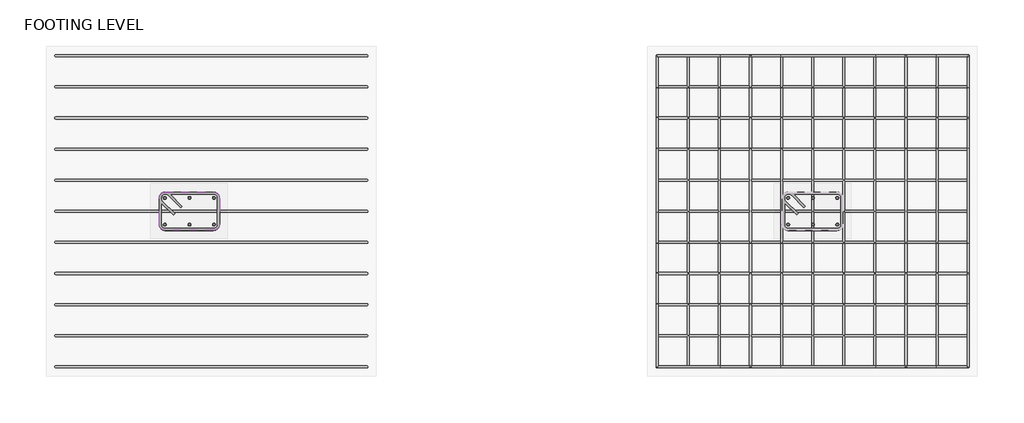
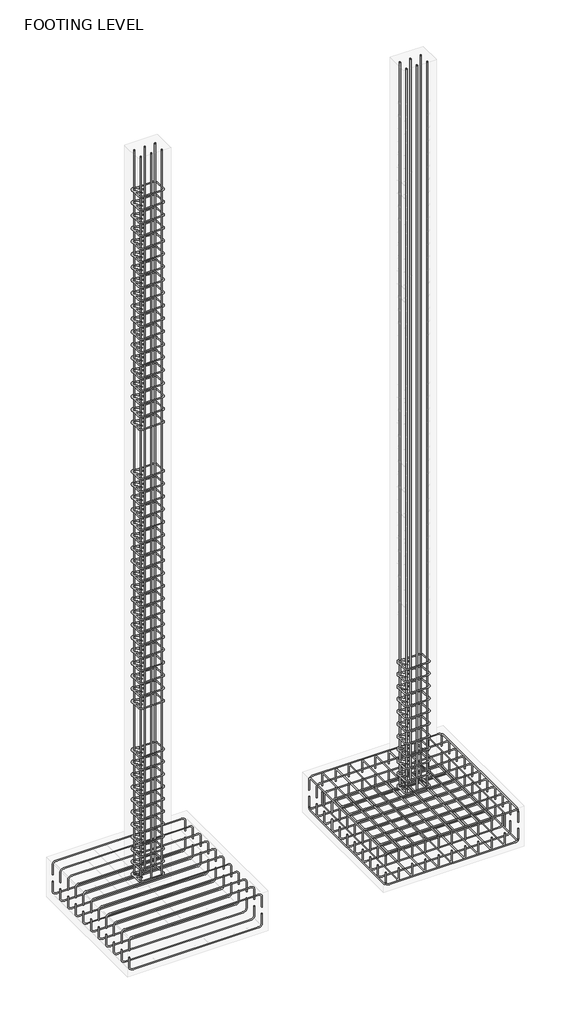
# One storey, part 8 of 9: 22 reinforcing bars.
"""IFC4 building model written with IfcOpenShell, lengths in millimetres."""

from ifc_helpers import new_model, si_unit, point, frame, origin, place, context, project, spatial, polyline, circle_curve, trimmed, segment, composite_curve, source, transform, mapped, element, save
from ifc_brep_helpers import swept_disk

model = new_model("IFC4")

# Units and contexts
model_context = context("Model", 3, world=origin())
ifc_project = project(units=[si_unit("LENGTHUNIT", "METRE", prefix="MILLI")], contexts=[model_context])

# Site, building, storey
site = spatial("IfcSite", under=ifc_project)
building = spatial("IfcBuilding", under=site)
storey = spatial("IfcBuildingStorey", under=building, Name="FOOTING LEVEL", Elevation=-1981.2)

# Reinforcing bars
placement = place(None, origin())
reinforcing_bar_shape = source(origin(), model_context, "Body", "SolidModel", [
    swept_disk(composite_curve([segment(polyline([(-6807.4208659, 8895.7158402, -2171.7), (-6807.4208659, 8895.7158402, -2057.4)]), True, "CONTINUOUS"), segment(trimmed(circle_curve(frame((-6774.0833659, 8895.7158402, -2057.4), z_axis=(0.0, 1.0, 0.0), x_axis=(-33.337499999999636, 0.0, 0.0)), 33.3375), [point((-6807.4208659, 8895.7158402, -2057.4))], [point((-6774.0833659, 8895.7158402, -2024.0625))], True, "CARTESIAN"), True, "CONTINUOUS"), segment(polyline([(-6774.0833659, 8895.7158402, -2024.0625), (-5402.4833659, 8895.7158402, -2024.0625)]), True, "CONTINUOUS"), segment(trimmed(circle_curve(frame((-5402.4833659, 8895.7158402, -2057.4), z_axis=(0.0, 1.0, 0.0), x_axis=(0.0, 0.0, 33.33750000000009)), 33.3375), [point((-5402.4833659, 8895.7158402, -2024.0625))], [point((-5369.1458659, 8895.7158402, -2057.4))], True, "CARTESIAN"), True, "CONTINUOUS"), segment(polyline([(-5369.1458659, 8895.7158402, -2057.4), (-5369.1458659, 8895.7158402, -2171.7)]), True, "CONTINUOUS")], self_intersect=False), 4.7625),
])
element("IfcReinforcingBar", 1, at=placement, inside=storey, context=model_context, shape_type="MappedRepresentation", body=[
    mapped(reinforcing_bar_shape, transform((0.0, 0.0, 0.0), x_axis=(1.0, 0.0, 0.0), y_axis=(0.0, 1.0, 0.0), z_axis=(0.0, 0.0, 1.0))),
    mapped(reinforcing_bar_shape, transform((0.0, -143.8275, 0.0), x_axis=(1.0, 0.0, 0.0), y_axis=(0.0, 1.0, 0.0), z_axis=(0.0, 0.0, 1.0))),
    mapped(reinforcing_bar_shape, transform((0.0, -287.655, 0.0), x_axis=(1.0, 0.0, 0.0), y_axis=(0.0, 1.0, 0.0), z_axis=(0.0, 0.0, 1.0))),
    mapped(reinforcing_bar_shape, transform((0.0, -431.4825, 0.0), x_axis=(1.0, 0.0, 0.0), y_axis=(0.0, 1.0, 0.0), z_axis=(0.0, 0.0, 1.0))),
    mapped(reinforcing_bar_shape, transform((0.0, -575.31, 0.0), x_axis=(1.0, 0.0, 0.0), y_axis=(0.0, 1.0, 0.0), z_axis=(0.0, 0.0, 1.0))),
    mapped(reinforcing_bar_shape, transform((0.0, -719.1375, 0.0), x_axis=(1.0, 0.0, 0.0), y_axis=(0.0, 1.0, 0.0), z_axis=(0.0, 0.0, 1.0))),
    mapped(reinforcing_bar_shape, transform((0.0, -862.965, 0.0), x_axis=(1.0, 0.0, 0.0), y_axis=(0.0, 1.0, 0.0), z_axis=(0.0, 0.0, 1.0))),
    mapped(reinforcing_bar_shape, transform((0.0, -1006.7925, 0.0), x_axis=(1.0, 0.0, 0.0), y_axis=(0.0, 1.0, 0.0), z_axis=(0.0, 0.0, 1.0))),
    mapped(reinforcing_bar_shape, transform((0.0, -1150.62, 0.0), x_axis=(1.0, 0.0, 0.0), y_axis=(0.0, 1.0, 0.0), z_axis=(0.0, 0.0, 1.0))),
    mapped(reinforcing_bar_shape, transform((0.0, -1294.4475, 0.0), x_axis=(1.0, 0.0, 0.0), y_axis=(0.0, 1.0, 0.0), z_axis=(0.0, 0.0, 1.0))),
    mapped(reinforcing_bar_shape, transform((0.0, -1438.275, 0.0), x_axis=(1.0, 0.0, 0.0), y_axis=(0.0, 1.0, 0.0), z_axis=(0.0, 0.0, 1.0))),
])
reinforcing_bar_2_shape = source(origin(), model_context, "Body", "SolidModel", [
    swept_disk(composite_curve([segment(polyline([(-6807.4208659, 7457.4408402, -2247.9), (-6807.4208659, 7457.4408402, -2362.2)]), True, "CONTINUOUS"), segment(trimmed(circle_curve(frame((-6774.0833659, 7457.4408402, -2362.2), z_axis=(0.0, -1.0, 0.0), x_axis=(-33.337499999999636, 0.0, 0.0)), 33.3375), [point((-6807.4208659, 7457.4408402, -2362.2))], [point((-6774.0833659, 7457.4408402, -2395.5375))], True, "CARTESIAN"), True, "CONTINUOUS"), segment(polyline([(-6774.0833659, 7457.4408402, -2395.5375), (-5402.4833659, 7457.4408402, -2395.5375)]), True, "CONTINUOUS"), segment(trimmed(circle_curve(frame((-5402.4833659, 7457.4408402, -2362.2), z_axis=(0.0, -1.0, 0.0), x_axis=(0.0, 0.0, -33.33750000000009)), 33.3375), [point((-5402.4833659, 7457.4408402, -2395.5375))], [point((-5369.1458659, 7457.4408402, -2362.2))], True, "CARTESIAN"), True, "CONTINUOUS"), segment(polyline([(-5369.1458659, 7457.4408402, -2362.2), (-5369.1458659, 7457.4408402, -2247.9)]), True, "CONTINUOUS")], self_intersect=False), 4.7625),
])
element("IfcReinforcingBar", 2, at=placement, inside=storey, context=model_context, shape_type="MappedRepresentation", body=[
    mapped(reinforcing_bar_2_shape, transform((0.0, 0.0, 0.0), x_axis=(1.0, 0.0, 0.0), y_axis=(0.0, 1.0, 0.0), z_axis=(0.0, 0.0, 1.0))),
    mapped(reinforcing_bar_2_shape, transform((0.0, 143.8275, 0.0), x_axis=(1.0, 0.0, 0.0), y_axis=(0.0, 1.0, 0.0), z_axis=(0.0, 0.0, 1.0))),
    mapped(reinforcing_bar_2_shape, transform((0.0, 287.655, 0.0), x_axis=(1.0, 0.0, 0.0), y_axis=(0.0, 1.0, 0.0), z_axis=(0.0, 0.0, 1.0))),
    mapped(reinforcing_bar_2_shape, transform((0.0, 431.4825, 0.0), x_axis=(1.0, 0.0, 0.0), y_axis=(0.0, 1.0, 0.0), z_axis=(0.0, 0.0, 1.0))),
    mapped(reinforcing_bar_2_shape, transform((0.0, 575.31, 0.0), x_axis=(1.0, 0.0, 0.0), y_axis=(0.0, 1.0, 0.0), z_axis=(0.0, 0.0, 1.0))),
    mapped(reinforcing_bar_2_shape, transform((0.0, 719.1375, 0.0), x_axis=(1.0, 0.0, 0.0), y_axis=(0.0, 1.0, 0.0), z_axis=(0.0, 0.0, 1.0))),
    mapped(reinforcing_bar_2_shape, transform((0.0, 862.965, 0.0), x_axis=(1.0, 0.0, 0.0), y_axis=(0.0, 1.0, 0.0), z_axis=(0.0, 0.0, 1.0))),
    mapped(reinforcing_bar_2_shape, transform((0.0, 1006.7925, 0.0), x_axis=(1.0, 0.0, 0.0), y_axis=(0.0, 1.0, 0.0), z_axis=(0.0, 0.0, 1.0))),
    mapped(reinforcing_bar_2_shape, transform((0.0, 1150.62, 0.0), x_axis=(1.0, 0.0, 0.0), y_axis=(0.0, 1.0, 0.0), z_axis=(0.0, 0.0, 1.0))),
    mapped(reinforcing_bar_2_shape, transform((0.0, 1294.4475, 0.0), x_axis=(1.0, 0.0, 0.0), y_axis=(0.0, 1.0, 0.0), z_axis=(0.0, 0.0, 1.0))),
    mapped(reinforcing_bar_2_shape, transform((0.0, 1438.275, 0.0), x_axis=(1.0, 0.0, 0.0), y_axis=(0.0, 1.0, 0.0), z_axis=(0.0, 0.0, 1.0))),
])
reinforcing_bar_3_shape = source(origin(), model_context, "Body", "SolidModel", [
    swept_disk(composite_curve([segment(polyline([(-2587.8458659, 8895.7158402, -2171.7), (-2587.8458659, 8895.7158402, -2057.4)]), True, "CONTINUOUS"), segment(trimmed(circle_curve(frame((-2587.8458659, 8862.3783402, -2057.4), z_axis=(1.0, 0.0, 0.0), x_axis=(0.0, 33.337499999999636, 0.0)), 33.3375), [point((-2587.8458659, 8895.7158402, -2057.4))], [point((-2587.8458659, 8862.3783402, -2024.0625))], True, "CARTESIAN"), True, "CONTINUOUS"), segment(polyline([(-2587.8458659, 8862.3783402, -2024.0625), (-2587.8458659, 7490.7783402, -2024.0625)]), True, "CONTINUOUS"), segment(trimmed(circle_curve(frame((-2587.8458659, 7490.7783402, -2057.4), z_axis=(1.0, 0.0, 0.0), x_axis=(0.0, 0.0, 33.33750000000009)), 33.3375), [point((-2587.8458659, 7490.7783402, -2024.0625))], [point((-2587.8458659, 7457.4408402, -2057.4))], True, "CARTESIAN"), True, "CONTINUOUS"), segment(polyline([(-2587.8458659, 7457.4408402, -2057.4), (-2587.8458659, 7457.4408402, -2171.7)]), True, "CONTINUOUS")], self_intersect=False), 4.7625),
])
element("IfcReinforcingBar", 3, at=placement, inside=storey, context=model_context, shape_type="MappedRepresentation", body=[
    mapped(reinforcing_bar_3_shape, transform((0.0, 0.0, 0.0), x_axis=(1.0, 0.0, 0.0), y_axis=(0.0, 1.0, 0.0), z_axis=(0.0, 0.0, 1.0))),
    mapped(reinforcing_bar_3_shape, transform((-143.8275, 0.0, 0.0), x_axis=(1.0, 0.0, 0.0), y_axis=(0.0, 1.0, 0.0), z_axis=(0.0, 0.0, 1.0))),
    mapped(reinforcing_bar_3_shape, transform((-287.655, 0.0, 0.0), x_axis=(1.0, 0.0, 0.0), y_axis=(0.0, 1.0, 0.0), z_axis=(0.0, 0.0, 1.0))),
    mapped(reinforcing_bar_3_shape, transform((-431.4825, 0.0, 0.0), x_axis=(1.0, 0.0, 0.0), y_axis=(0.0, 1.0, 0.0), z_axis=(0.0, 0.0, 1.0))),
    mapped(reinforcing_bar_3_shape, transform((-575.31, 0.0, 0.0), x_axis=(1.0, 0.0, 0.0), y_axis=(0.0, 1.0, 0.0), z_axis=(0.0, 0.0, 1.0))),
    mapped(reinforcing_bar_3_shape, transform((-719.1375, 0.0, 0.0), x_axis=(1.0, 0.0, 0.0), y_axis=(0.0, 1.0, 0.0), z_axis=(0.0, 0.0, 1.0))),
    mapped(reinforcing_bar_3_shape, transform((-862.965, 0.0, 0.0), x_axis=(1.0, 0.0, 0.0), y_axis=(0.0, 1.0, 0.0), z_axis=(0.0, 0.0, 1.0))),
    mapped(reinforcing_bar_3_shape, transform((-1006.7925, 0.0, 0.0), x_axis=(1.0, 0.0, 0.0), y_axis=(0.0, 1.0, 0.0), z_axis=(0.0, 0.0, 1.0))),
    mapped(reinforcing_bar_3_shape, transform((-1150.62, 0.0, 0.0), x_axis=(1.0, 0.0, 0.0), y_axis=(0.0, 1.0, 0.0), z_axis=(0.0, 0.0, 1.0))),
    mapped(reinforcing_bar_3_shape, transform((-1294.4475, 0.0, 0.0), x_axis=(1.0, 0.0, 0.0), y_axis=(0.0, 1.0, 0.0), z_axis=(0.0, 0.0, 1.0))),
    mapped(reinforcing_bar_3_shape, transform((-1438.275, 0.0, 0.0), x_axis=(1.0, 0.0, 0.0), y_axis=(0.0, 1.0, 0.0), z_axis=(0.0, 0.0, 1.0))),
])
reinforcing_bar_4_shape = source(origin(), model_context, "Body", "SolidModel", [
    swept_disk(composite_curve([segment(polyline([(-2587.8458659, 7457.4408402, -2247.9), (-2587.8458659, 7457.4408402, -2362.2)]), True, "CONTINUOUS"), segment(trimmed(circle_curve(frame((-2587.8458659, 7490.7783402, -2362.2), z_axis=(1.0, 0.0, 0.0), x_axis=(0.0, -33.337499999999636, 0.0)), 33.3375), [point((-2587.8458659, 7457.4408402, -2362.2))], [point((-2587.8458659, 7490.7783402, -2395.5375))], True, "CARTESIAN"), True, "CONTINUOUS"), segment(polyline([(-2587.8458659, 7490.7783402, -2395.5375), (-2587.8458659, 8862.3783402, -2395.5375)]), True, "CONTINUOUS"), segment(trimmed(circle_curve(frame((-2587.8458659, 8862.3783402, -2362.2), z_axis=(1.0, 0.0, 0.0), x_axis=(0.0, 0.0, -33.33750000000009)), 33.3375), [point((-2587.8458659, 8862.3783402, -2395.5375))], [point((-2587.8458659, 8895.7158402, -2362.2))], True, "CARTESIAN"), True, "CONTINUOUS"), segment(polyline([(-2587.8458659, 8895.7158402, -2362.2), (-2587.8458659, 8895.7158402, -2247.9)]), True, "CONTINUOUS")], self_intersect=False), 4.7625),
])
element("IfcReinforcingBar", 4, at=placement, inside=storey, context=model_context, shape_type="MappedRepresentation", body=[
    mapped(reinforcing_bar_4_shape, transform((0.0, 0.0, 0.0), x_axis=(1.0, 0.0, 0.0), y_axis=(0.0, 1.0, 0.0), z_axis=(0.0, 0.0, 1.0))),
    mapped(reinforcing_bar_4_shape, transform((-143.8275, 0.0, 0.0), x_axis=(1.0, 0.0, 0.0), y_axis=(0.0, 1.0, 0.0), z_axis=(0.0, 0.0, 1.0))),
    mapped(reinforcing_bar_4_shape, transform((-287.655, 0.0, 0.0), x_axis=(1.0, 0.0, 0.0), y_axis=(0.0, 1.0, 0.0), z_axis=(0.0, 0.0, 1.0))),
    mapped(reinforcing_bar_4_shape, transform((-431.4825, 0.0, 0.0), x_axis=(1.0, 0.0, 0.0), y_axis=(0.0, 1.0, 0.0), z_axis=(0.0, 0.0, 1.0))),
    mapped(reinforcing_bar_4_shape, transform((-575.31, 0.0, 0.0), x_axis=(1.0, 0.0, 0.0), y_axis=(0.0, 1.0, 0.0), z_axis=(0.0, 0.0, 1.0))),
    mapped(reinforcing_bar_4_shape, transform((-719.1375, 0.0, 0.0), x_axis=(1.0, 0.0, 0.0), y_axis=(0.0, 1.0, 0.0), z_axis=(0.0, 0.0, 1.0))),
    mapped(reinforcing_bar_4_shape, transform((-862.965, 0.0, 0.0), x_axis=(1.0, 0.0, 0.0), y_axis=(0.0, 1.0, 0.0), z_axis=(0.0, 0.0, 1.0))),
    mapped(reinforcing_bar_4_shape, transform((-1006.7925, 0.0, 0.0), x_axis=(1.0, 0.0, 0.0), y_axis=(0.0, 1.0, 0.0), z_axis=(0.0, 0.0, 1.0))),
    mapped(reinforcing_bar_4_shape, transform((-1150.62, 0.0, 0.0), x_axis=(1.0, 0.0, 0.0), y_axis=(0.0, 1.0, 0.0), z_axis=(0.0, 0.0, 1.0))),
    mapped(reinforcing_bar_4_shape, transform((-1294.4475, 0.0, 0.0), x_axis=(1.0, 0.0, 0.0), y_axis=(0.0, 1.0, 0.0), z_axis=(0.0, 0.0, 1.0))),
    mapped(reinforcing_bar_4_shape, transform((-1438.275, 0.0, 0.0), x_axis=(1.0, 0.0, 0.0), y_axis=(0.0, 1.0, 0.0), z_axis=(0.0, 0.0, 1.0))),
])
reinforcing_bar_5_shape = source(origin(), model_context, "Body", "SolidModel", [
    swept_disk(composite_curve([segment(polyline([(-4026.1208659, 8895.7158402, -2171.7), (-4026.1208659, 8895.7158402, -2057.4)]), True, "CONTINUOUS"), segment(trimmed(circle_curve(frame((-3992.7833659, 8895.7158402, -2057.4), z_axis=(0.0, 1.0, 0.0), x_axis=(-33.33750000000009, 0.0, 0.0)), 33.3375), [point((-4026.1208659, 8895.7158402, -2057.4))], [point((-3992.7833659, 8895.7158402, -2024.0625))], True, "CARTESIAN"), True, "CONTINUOUS"), segment(polyline([(-3992.7833659, 8895.7158402, -2024.0625), (-2621.1833659, 8895.7158402, -2024.0625)]), True, "CONTINUOUS"), segment(trimmed(circle_curve(frame((-2621.1833659, 8895.7158402, -2057.4), z_axis=(0.0, 1.0, 0.0), x_axis=(0.0, 0.0, 33.33750000000009)), 33.3375), [point((-2621.1833659, 8895.7158402, -2024.0625))], [point((-2587.8458659, 8895.7158402, -2057.4))], True, "CARTESIAN"), True, "CONTINUOUS"), segment(polyline([(-2587.8458659, 8895.7158402, -2057.4), (-2587.8458659, 8895.7158402, -2171.7)]), True, "CONTINUOUS")], self_intersect=False), 4.7625),
])
element("IfcReinforcingBar", 5, at=placement, inside=storey, context=model_context, shape_type="MappedRepresentation", body=[
    mapped(reinforcing_bar_5_shape, transform((0.0, 0.0, 0.0), x_axis=(1.0, 0.0, 0.0), y_axis=(0.0, 1.0, 0.0), z_axis=(0.0, 0.0, 1.0))),
    mapped(reinforcing_bar_5_shape, transform((0.0, -143.8275, 0.0), x_axis=(1.0, 0.0, 0.0), y_axis=(0.0, 1.0, 0.0), z_axis=(0.0, 0.0, 1.0))),
    mapped(reinforcing_bar_5_shape, transform((0.0, -287.655, 0.0), x_axis=(1.0, 0.0, 0.0), y_axis=(0.0, 1.0, 0.0), z_axis=(0.0, 0.0, 1.0))),
    mapped(reinforcing_bar_5_shape, transform((0.0, -431.4825, 0.0), x_axis=(1.0, 0.0, 0.0), y_axis=(0.0, 1.0, 0.0), z_axis=(0.0, 0.0, 1.0))),
    mapped(reinforcing_bar_5_shape, transform((0.0, -575.31, 0.0), x_axis=(1.0, 0.0, 0.0), y_axis=(0.0, 1.0, 0.0), z_axis=(0.0, 0.0, 1.0))),
    mapped(reinforcing_bar_5_shape, transform((0.0, -719.1375, 0.0), x_axis=(1.0, 0.0, 0.0), y_axis=(0.0, 1.0, 0.0), z_axis=(0.0, 0.0, 1.0))),
    mapped(reinforcing_bar_5_shape, transform((0.0, -862.965, 0.0), x_axis=(1.0, 0.0, 0.0), y_axis=(0.0, 1.0, 0.0), z_axis=(0.0, 0.0, 1.0))),
    mapped(reinforcing_bar_5_shape, transform((0.0, -1006.7925, 0.0), x_axis=(1.0, 0.0, 0.0), y_axis=(0.0, 1.0, 0.0), z_axis=(0.0, 0.0, 1.0))),
    mapped(reinforcing_bar_5_shape, transform((0.0, -1150.62, 0.0), x_axis=(1.0, 0.0, 0.0), y_axis=(0.0, 1.0, 0.0), z_axis=(0.0, 0.0, 1.0))),
    mapped(reinforcing_bar_5_shape, transform((0.0, -1294.4475, 0.0), x_axis=(1.0, 0.0, 0.0), y_axis=(0.0, 1.0, 0.0), z_axis=(0.0, 0.0, 1.0))),
    mapped(reinforcing_bar_5_shape, transform((0.0, -1438.275, 0.0), x_axis=(1.0, 0.0, 0.0), y_axis=(0.0, 1.0, 0.0), z_axis=(0.0, 0.0, 1.0))),
])
reinforcing_bar_6_shape = source(origin(), model_context, "Body", "SolidModel", [
    swept_disk(composite_curve([segment(polyline([(-4026.1208659, 7457.4408402, -2247.9), (-4026.1208659, 7457.4408402, -2362.2)]), True, "CONTINUOUS"), segment(trimmed(circle_curve(frame((-3992.7833659, 7457.4408402, -2362.2), z_axis=(0.0, -1.0, 0.0), x_axis=(-33.33750000000009, 0.0, 0.0)), 33.3375), [point((-4026.1208659, 7457.4408402, -2362.2))], [point((-3992.7833659, 7457.4408402, -2395.5375))], True, "CARTESIAN"), True, "CONTINUOUS"), segment(polyline([(-3992.7833659, 7457.4408402, -2395.5375), (-2621.1833659, 7457.4408402, -2395.5375)]), True, "CONTINUOUS"), segment(trimmed(circle_curve(frame((-2621.1833659, 7457.4408402, -2362.2), z_axis=(0.0, -1.0, 0.0), x_axis=(0.0, 0.0, -33.33750000000009)), 33.3375), [point((-2621.1833659, 7457.4408402, -2395.5375))], [point((-2587.8458659, 7457.4408402, -2362.2))], True, "CARTESIAN"), True, "CONTINUOUS"), segment(polyline([(-2587.8458659, 7457.4408402, -2362.2), (-2587.8458659, 7457.4408402, -2247.9)]), True, "CONTINUOUS")], self_intersect=False), 4.7625),
])
element("IfcReinforcingBar", 6, at=placement, inside=storey, context=model_context, shape_type="MappedRepresentation", body=[
    mapped(reinforcing_bar_6_shape, transform((0.0, 0.0, 0.0), x_axis=(1.0, 0.0, 0.0), y_axis=(0.0, 1.0, 0.0), z_axis=(0.0, 0.0, 1.0))),
    mapped(reinforcing_bar_6_shape, transform((0.0, 143.8275, 0.0), x_axis=(1.0, 0.0, 0.0), y_axis=(0.0, 1.0, 0.0), z_axis=(0.0, 0.0, 1.0))),
    mapped(reinforcing_bar_6_shape, transform((0.0, 287.655, 0.0), x_axis=(1.0, 0.0, 0.0), y_axis=(0.0, 1.0, 0.0), z_axis=(0.0, 0.0, 1.0))),
    mapped(reinforcing_bar_6_shape, transform((0.0, 431.4825, 0.0), x_axis=(1.0, 0.0, 0.0), y_axis=(0.0, 1.0, 0.0), z_axis=(0.0, 0.0, 1.0))),
    mapped(reinforcing_bar_6_shape, transform((0.0, 575.31, 0.0), x_axis=(1.0, 0.0, 0.0), y_axis=(0.0, 1.0, 0.0), z_axis=(0.0, 0.0, 1.0))),
    mapped(reinforcing_bar_6_shape, transform((0.0, 719.1375, 0.0), x_axis=(1.0, 0.0, 0.0), y_axis=(0.0, 1.0, 0.0), z_axis=(0.0, 0.0, 1.0))),
    mapped(reinforcing_bar_6_shape, transform((0.0, 862.965, 0.0), x_axis=(1.0, 0.0, 0.0), y_axis=(0.0, 1.0, 0.0), z_axis=(0.0, 0.0, 1.0))),
    mapped(reinforcing_bar_6_shape, transform((0.0, 1006.7925, 0.0), x_axis=(1.0, 0.0, 0.0), y_axis=(0.0, 1.0, 0.0), z_axis=(0.0, 0.0, 1.0))),
    mapped(reinforcing_bar_6_shape, transform((0.0, 1150.62, 0.0), x_axis=(1.0, 0.0, 0.0), y_axis=(0.0, 1.0, 0.0), z_axis=(0.0, 0.0, 1.0))),
    mapped(reinforcing_bar_6_shape, transform((0.0, 1294.4475, 0.0), x_axis=(1.0, 0.0, 0.0), y_axis=(0.0, 1.0, 0.0), z_axis=(0.0, 0.0, 1.0))),
    mapped(reinforcing_bar_6_shape, transform((0.0, 1438.275, 0.0), x_axis=(1.0, 0.0, 0.0), y_axis=(0.0, 1.0, 0.0), z_axis=(0.0, 0.0, 1.0))),
])
reinforcing_bar_7_shape = source(origin(), model_context, "Body", "SolidModel", [
    swept_disk(composite_curve([segment(polyline([(-6227.3061886, 8196.8771233, -1938.3375), (-6284.1703857, 8253.7413204, -1938.3375)]), True, "CONTINUOUS"), segment(trimmed(circle_curve(frame((-6301.0083659, 8236.9033402, -1938.3375), z_axis=(0.0, 0.0, 1.0), x_axis=(16.837980199999947, 16.837980199999947, 0.0)), 23.8125), [point((-6284.1703857, 8253.7413204, -1938.3375))], [point((-6324.8208659, 8236.9033402, -1938.3375))], True, "CARTESIAN"), True, "CONTINUOUS"), segment(polyline([(-6324.8208659, 8236.9033402, -1938.3375), (-6324.8208659, 8116.2533402, -1938.3375)]), True, "CONTINUOUS"), segment(trimmed(circle_curve(frame((-6301.0083659, 8116.2533402, -1938.3375), z_axis=(0.0, 0.0, 1.0), x_axis=(-23.8125, 0.0, 0.0)), 23.8125), [point((-6324.8208659, 8116.2533402, -1938.3375))], [point((-6301.0083659, 8092.4408402, -1938.3375))], True, "CARTESIAN"), True, "CONTINUOUS"), segment(polyline([(-6301.0083659, 8092.4408402, -1938.3375), (-6078.7583659, 8092.4408402, -1938.3375)]), True, "CONTINUOUS"), segment(trimmed(circle_curve(frame((-6078.7583659, 8116.2152841, -1939.6832232), z_axis=(0.0, 0.056513312022656255, 0.9984018457335854), x_axis=(0.0, -23.774443899999824, 1.3457231999998385)), 23.8125), [point((-6078.7583659, 8092.4408402, -1938.3375))], [point((-6054.9458659, 8116.2152841, -1939.6832232))], True, "CARTESIAN"), True, "CONTINUOUS"), segment(polyline([(-6054.9458659, 8116.2152841, -1939.6832232), (-6054.9458659, 8236.9413962, -1946.5167768)]), True, "CONTINUOUS"), segment(trimmed(circle_curve(frame((-6078.7583659, 8236.9413962, -1946.5167768), z_axis=(0.0, 0.056513312022656255, 0.9984018457335854), x_axis=(23.8125, 0.0, 0.0)), 23.8125), [point((-6054.9458659, 8236.9413962, -1946.5167768))], [point((-6078.7583659, 8260.7158402, -1947.8625))], True, "CARTESIAN"), True, "CONTINUOUS"), segment(polyline([(-6078.7583659, 8260.7158402, -1947.8625), (-6301.0083659, 8260.7158402, -1947.8625)]), True, "CONTINUOUS"), segment(trimmed(circle_curve(frame((-6301.0083659, 8236.9033402, -1947.8625), z_axis=(0.0, 0.0, 1.0), x_axis=(0.0, 23.8125, 0.0)), 23.8125), [point((-6301.0083659, 8260.7158402, -1947.8625))], [point((-6317.8463461, 8220.06536, -1947.8625))], True, "CARTESIAN"), True, "CONTINUOUS"), segment(polyline([(-6317.8463461, 8220.06536, -1947.8625), (-6260.9821491, 8163.2011629, -1947.8625)]), True, "CONTINUOUS")], self_intersect=False), 4.7625),
])
element("IfcReinforcingBar", 7, at=placement, inside=storey, context=model_context, shape_type="MappedRepresentation", body=[
    mapped(reinforcing_bar_7_shape, transform((0.0, 0.0, 0.0), x_axis=(1.0, 0.0, 0.0), y_axis=(0.0, 1.0, 0.0), z_axis=(0.0, 0.0, 1.0))),
    mapped(reinforcing_bar_7_shape, transform((0.0, 0.0, 142.5866456), x_axis=(1.0, 0.0, 0.0), y_axis=(0.0, 1.0, 0.0), z_axis=(0.0, 0.0, 1.0))),
    mapped(reinforcing_bar_7_shape, transform((0.0, 0.0, 285.1732912), x_axis=(1.0, 0.0, 0.0), y_axis=(0.0, 1.0, 0.0), z_axis=(0.0, 0.0, 1.0))),
    mapped(reinforcing_bar_7_shape, transform((0.0, 0.0, 427.7599369), x_axis=(1.0, 0.0, 0.0), y_axis=(0.0, 1.0, 0.0), z_axis=(0.0, 0.0, 1.0))),
    mapped(reinforcing_bar_7_shape, transform((0.0, 0.0, 570.3465825), x_axis=(1.0, 0.0, 0.0), y_axis=(0.0, 1.0, 0.0), z_axis=(0.0, 0.0, 1.0))),
    mapped(reinforcing_bar_7_shape, transform((0.0, 0.0, 712.9332281), x_axis=(1.0, 0.0, 0.0), y_axis=(0.0, 1.0, 0.0), z_axis=(0.0, 0.0, 1.0))),
    mapped(reinforcing_bar_7_shape, transform((0.0, 0.0, 855.5198737), x_axis=(1.0, 0.0, 0.0), y_axis=(0.0, 1.0, 0.0), z_axis=(0.0, 0.0, 1.0))),
    mapped(reinforcing_bar_7_shape, transform((0.0, 0.0, 998.1065193), x_axis=(1.0, 0.0, 0.0), y_axis=(0.0, 1.0, 0.0), z_axis=(0.0, 0.0, 1.0))),
    mapped(reinforcing_bar_7_shape, transform((0.0, 0.0, 1140.6931649), x_axis=(1.0, 0.0, 0.0), y_axis=(0.0, 1.0, 0.0), z_axis=(0.0, 0.0, 1.0))),
    mapped(reinforcing_bar_7_shape, transform((0.0, 0.0, 1283.2798106), x_axis=(1.0, 0.0, 0.0), y_axis=(0.0, 1.0, 0.0), z_axis=(0.0, 0.0, 1.0))),
    mapped(reinforcing_bar_7_shape, transform((0.0, 0.0, 1425.8664562), x_axis=(1.0, 0.0, 0.0), y_axis=(0.0, 1.0, 0.0), z_axis=(0.0, 0.0, 1.0))),
])
element("IfcReinforcingBar", 8, at=placement, inside=storey, context=model_context, shape_type="SolidModel", body=[
    swept_disk(composite_curve([segment(polyline([(-6076.4020268, 8238.383248, -1943.1), (-6076.4020268, 8238.383248, 6362.7)]), True, "CONTINUOUS")], self_intersect=False), 6.35),
])
element("IfcReinforcingBar", 9, at=placement, inside=storey, context=model_context, shape_type="SolidModel", body=[
    swept_disk(composite_curve([segment(polyline([(-6076.4020268, 8114.7734324, -1943.1), (-6076.4020268, 8114.7734324, 6362.7)]), True, "CONTINUOUS")], self_intersect=False), 6.35),
])
element("IfcReinforcingBar", 10, at=placement, inside=storey, context=model_context, shape_type="SolidModel", body=[
    swept_disk(composite_curve([segment(polyline([(-6303.364705, 8238.383248, -1943.1), (-6303.364705, 8238.383248, 6362.7)]), True, "CONTINUOUS")], self_intersect=False), 6.35),
])
element("IfcReinforcingBar", 11, at=placement, inside=storey, context=model_context, shape_type="SolidModel", body=[
    swept_disk(composite_curve([segment(polyline([(-6303.364705, 8114.7734324, -1943.1), (-6303.364705, 8114.7734324, 6362.7)]), True, "CONTINUOUS")], self_intersect=False), 6.35),
])
element("IfcReinforcingBar", 12, at=placement, inside=storey, context=model_context, shape_type="SolidModel", body=[
    swept_disk(composite_curve([segment(polyline([(-6189.064705, 8238.383248, -1943.1), (-6189.064705, 8238.383248, 6362.7)]), True, "CONTINUOUS")], self_intersect=False), 6.35),
])
element("IfcReinforcingBar", 13, at=placement, inside=storey, context=model_context, shape_type="SolidModel", body=[
    swept_disk(composite_curve([segment(polyline([(-6189.064705, 8114.7734324, -1943.1), (-6189.064705, 8114.7734324, 6362.7)]), True, "CONTINUOUS")], self_intersect=False), 6.35),
])
reinforcing_bar_8_shape = source(origin(), model_context, "Body", "SolidModel", [
    swept_disk(composite_curve([segment(polyline([(-3344.4061886, 8196.8771233, -1938.3375), (-3401.2703857, 8253.7413204, -1938.3375)]), True, "CONTINUOUS"), segment(trimmed(circle_curve(frame((-3418.1083659, 8236.9033402, -1938.3375), z_axis=(0.0, 0.0, 1.0), x_axis=(16.837980199999947, 16.837980199999947, 0.0)), 23.8125), [point((-3401.2703857, 8253.7413204, -1938.3375))], [point((-3441.9208659, 8236.9033402, -1938.3375))], True, "CARTESIAN"), True, "CONTINUOUS"), segment(polyline([(-3441.9208659, 8236.9033402, -1938.3375), (-3441.9208659, 8116.2533402, -1938.3375)]), True, "CONTINUOUS"), segment(trimmed(circle_curve(frame((-3418.1083659, 8116.2533402, -1938.3375), z_axis=(0.0, 0.0, 1.0), x_axis=(-23.8125, 0.0, 0.0)), 23.8125), [point((-3441.9208659, 8116.2533402, -1938.3375))], [point((-3418.1083659, 8092.4408402, -1938.3375))], True, "CARTESIAN"), True, "CONTINUOUS"), segment(polyline([(-3418.1083659, 8092.4408402, -1938.3375), (-3195.8583659, 8092.4408402, -1938.3375)]), True, "CONTINUOUS"), segment(trimmed(circle_curve(frame((-3195.8583659, 8116.2152841, -1939.6832232), z_axis=(0.0, 0.056513312022656255, 0.9984018457335854), x_axis=(0.0, -23.774443899999824, 1.3457231999998385)), 23.8125), [point((-3195.8583659, 8092.4408402, -1938.3375))], [point((-3172.0458659, 8116.2152841, -1939.6832232))], True, "CARTESIAN"), True, "CONTINUOUS"), segment(polyline([(-3172.0458659, 8116.2152841, -1939.6832232), (-3172.0458659, 8236.9413962, -1946.5167768)]), True, "CONTINUOUS"), segment(trimmed(circle_curve(frame((-3195.8583659, 8236.9413962, -1946.5167768), z_axis=(0.0, 0.056513312022656255, 0.9984018457335854), x_axis=(23.8125, 0.0, 0.0)), 23.8125), [point((-3172.0458659, 8236.9413962, -1946.5167768))], [point((-3195.8583659, 8260.7158402, -1947.8625))], True, "CARTESIAN"), True, "CONTINUOUS"), segment(polyline([(-3195.8583659, 8260.7158402, -1947.8625), (-3418.1083659, 8260.7158402, -1947.8625)]), True, "CONTINUOUS"), segment(trimmed(circle_curve(frame((-3418.1083659, 8236.9033402, -1947.8625), z_axis=(0.0, 0.0, 1.0), x_axis=(0.0, 23.8125, 0.0)), 23.8125), [point((-3418.1083659, 8260.7158402, -1947.8625))], [point((-3434.9463461, 8220.06536, -1947.8625))], True, "CARTESIAN"), True, "CONTINUOUS"), segment(polyline([(-3434.9463461, 8220.06536, -1947.8625), (-3378.0821491, 8163.2011629, -1947.8625)]), True, "CONTINUOUS")], self_intersect=False), 4.7625),
])
element("IfcReinforcingBar", 14, at=placement, inside=storey, context=model_context, shape_type="MappedRepresentation", body=[
    mapped(reinforcing_bar_8_shape, transform((0.0, 0.0, 0.0), x_axis=(1.0, 0.0, 0.0), y_axis=(0.0, 1.0, 0.0), z_axis=(0.0, 0.0, 1.0))),
    mapped(reinforcing_bar_8_shape, transform((0.0, 0.0, 142.5866456), x_axis=(1.0, 0.0, 0.0), y_axis=(0.0, 1.0, 0.0), z_axis=(0.0, 0.0, 1.0))),
    mapped(reinforcing_bar_8_shape, transform((0.0, 0.0, 285.1732912), x_axis=(1.0, 0.0, 0.0), y_axis=(0.0, 1.0, 0.0), z_axis=(0.0, 0.0, 1.0))),
    mapped(reinforcing_bar_8_shape, transform((0.0, 0.0, 427.7599369), x_axis=(1.0, 0.0, 0.0), y_axis=(0.0, 1.0, 0.0), z_axis=(0.0, 0.0, 1.0))),
    mapped(reinforcing_bar_8_shape, transform((0.0, 0.0, 570.3465825), x_axis=(1.0, 0.0, 0.0), y_axis=(0.0, 1.0, 0.0), z_axis=(0.0, 0.0, 1.0))),
    mapped(reinforcing_bar_8_shape, transform((0.0, 0.0, 712.9332281), x_axis=(1.0, 0.0, 0.0), y_axis=(0.0, 1.0, 0.0), z_axis=(0.0, 0.0, 1.0))),
    mapped(reinforcing_bar_8_shape, transform((0.0, 0.0, 855.5198737), x_axis=(1.0, 0.0, 0.0), y_axis=(0.0, 1.0, 0.0), z_axis=(0.0, 0.0, 1.0))),
    mapped(reinforcing_bar_8_shape, transform((0.0, 0.0, 998.1065193), x_axis=(1.0, 0.0, 0.0), y_axis=(0.0, 1.0, 0.0), z_axis=(0.0, 0.0, 1.0))),
    mapped(reinforcing_bar_8_shape, transform((0.0, 0.0, 1140.6931649), x_axis=(1.0, 0.0, 0.0), y_axis=(0.0, 1.0, 0.0), z_axis=(0.0, 0.0, 1.0))),
    mapped(reinforcing_bar_8_shape, transform((0.0, 0.0, 1283.2798106), x_axis=(1.0, 0.0, 0.0), y_axis=(0.0, 1.0, 0.0), z_axis=(0.0, 0.0, 1.0))),
    mapped(reinforcing_bar_8_shape, transform((0.0, 0.0, 1425.8664562), x_axis=(1.0, 0.0, 0.0), y_axis=(0.0, 1.0, 0.0), z_axis=(0.0, 0.0, 1.0))),
])
element("IfcReinforcingBar", 15, at=placement, inside=storey, context=model_context, shape_type="SolidModel", body=[
    swept_disk(composite_curve([segment(polyline([(-3193.5020268, 8238.383248, -1943.1), (-3193.5020268, 8238.383248, 6362.7)]), True, "CONTINUOUS")], self_intersect=False), 6.35),
])
element("IfcReinforcingBar", 16, at=placement, inside=storey, context=model_context, shape_type="SolidModel", body=[
    swept_disk(composite_curve([segment(polyline([(-3193.5020268, 8114.7734324, -1943.1), (-3193.5020268, 8114.7734324, 6362.7)]), True, "CONTINUOUS")], self_intersect=False), 6.35),
])
element("IfcReinforcingBar", 17, at=placement, inside=storey, context=model_context, shape_type="SolidModel", body=[
    swept_disk(composite_curve([segment(polyline([(-3420.464705, 8238.383248, -1943.1), (-3420.464705, 8238.383248, 6362.7)]), True, "CONTINUOUS")], self_intersect=False), 6.35),
])
element("IfcReinforcingBar", 18, at=placement, inside=storey, context=model_context, shape_type="SolidModel", body=[
    swept_disk(composite_curve([segment(polyline([(-3420.464705, 8114.7734324, -1943.1), (-3420.464705, 8114.7734324, 6362.7)]), True, "CONTINUOUS")], self_intersect=False), 6.35),
])
element("IfcReinforcingBar", 19, at=placement, inside=storey, context=model_context, shape_type="SolidModel", body=[
    swept_disk(composite_curve([segment(polyline([(-3306.164705, 8238.383248, -1943.1), (-3306.164705, 8238.383248, 6362.7)]), True, "CONTINUOUS")], self_intersect=False), 6.35),
])
element("IfcReinforcingBar", 20, at=placement, inside=storey, context=model_context, shape_type="SolidModel", body=[
    swept_disk(composite_curve([segment(polyline([(-3306.164705, 8114.7734324, -1943.1), (-3306.164705, 8114.7734324, 6362.7)]), True, "CONTINUOUS")], self_intersect=False), 6.35),
])
reinforcing_bar_9_shape = source(origin(), model_context, "Body", "SolidModel", [
    swept_disk(composite_curve([segment(polyline([(-6227.3061886, 8196.8771233, 42.8625), (-6284.1703857, 8253.7413204, 42.8625)]), True, "CONTINUOUS"), segment(trimmed(circle_curve(frame((-6301.0083659, 8236.9033402, 42.8625), z_axis=(0.0, 0.0, 1.0), x_axis=(16.837980199999947, 16.837980199999947, 0.0)), 23.8125), [point((-6284.1703857, 8253.7413204, 42.8625))], [point((-6324.8208659, 8236.9033402, 42.8625))], True, "CARTESIAN"), True, "CONTINUOUS"), segment(polyline([(-6324.8208659, 8236.9033402, 42.8625), (-6324.8208659, 8116.2533402, 42.8625)]), True, "CONTINUOUS"), segment(trimmed(circle_curve(frame((-6301.0083659, 8116.2533402, 42.8625), z_axis=(0.0, 0.0, 1.0), x_axis=(-23.8125, 0.0, 0.0)), 23.8125), [point((-6324.8208659, 8116.2533402, 42.8625))], [point((-6301.0083659, 8092.4408402, 42.8625))], True, "CARTESIAN"), True, "CONTINUOUS"), segment(polyline([(-6301.0083659, 8092.4408402, 42.8625), (-6078.7583659, 8092.4408402, 42.8625)]), True, "CONTINUOUS"), segment(trimmed(circle_curve(frame((-6078.7583659, 8116.2152841, 41.5167768), z_axis=(0.0, 0.056513312022656255, 0.9984018457335854), x_axis=(0.0, -23.774443899999824, 1.3457231999999948)), 23.8125), [point((-6078.7583659, 8092.4408402, 42.8625))], [point((-6054.9458659, 8116.2152841, 41.5167768))], True, "CARTESIAN"), True, "CONTINUOUS"), segment(polyline([(-6054.9458659, 8116.2152841, 41.5167768), (-6054.9458659, 8236.9413962, 34.6832232)]), True, "CONTINUOUS"), segment(trimmed(circle_curve(frame((-6078.7583659, 8236.9413962, 34.6832232), z_axis=(0.0, 0.056513312022656255, 0.9984018457335854), x_axis=(23.8125, 0.0, 0.0)), 23.8125), [point((-6054.9458659, 8236.9413962, 34.6832232))], [point((-6078.7583659, 8260.7158402, 33.3375))], True, "CARTESIAN"), True, "CONTINUOUS"), segment(polyline([(-6078.7583659, 8260.7158402, 33.3375), (-6301.0083659, 8260.7158402, 33.3375)]), True, "CONTINUOUS"), segment(trimmed(circle_curve(frame((-6301.0083659, 8236.9033402, 33.3375), z_axis=(0.0, 0.0, 1.0), x_axis=(0.0, 23.8125, 0.0)), 23.8125), [point((-6301.0083659, 8260.7158402, 33.3375))], [point((-6317.8463461, 8220.06536, 33.3375))], True, "CARTESIAN"), True, "CONTINUOUS"), segment(polyline([(-6317.8463461, 8220.06536, 33.3375), (-6260.9821491, 8163.2011629, 33.3375)]), True, "CONTINUOUS")], self_intersect=False), 4.7625),
])
element("IfcReinforcingBar", 21, at=placement, inside=storey, context=model_context, shape_type="MappedRepresentation", body=[
    mapped(reinforcing_bar_9_shape, transform((0.0, 0.0, 0.0), x_axis=(1.0, 0.0, 0.0), y_axis=(0.0, 1.0, 0.0), z_axis=(0.0, 0.0, 1.0))),
    mapped(reinforcing_bar_9_shape, transform((0.0, 0.0, 146.5540169), x_axis=(1.0, 0.0, 0.0), y_axis=(0.0, 1.0, 0.0), z_axis=(0.0, 0.0, 1.0))),
    mapped(reinforcing_bar_9_shape, transform((0.0, 0.0, 293.1080338), x_axis=(1.0, 0.0, 0.0), y_axis=(0.0, 1.0, 0.0), z_axis=(0.0, 0.0, 1.0))),
    mapped(reinforcing_bar_9_shape, transform((0.0, 0.0, 439.6620507), x_axis=(1.0, 0.0, 0.0), y_axis=(0.0, 1.0, 0.0), z_axis=(0.0, 0.0, 1.0))),
    mapped(reinforcing_bar_9_shape, transform((0.0, 0.0, 586.2160676), x_axis=(1.0, 0.0, 0.0), y_axis=(0.0, 1.0, 0.0), z_axis=(0.0, 0.0, 1.0))),
    mapped(reinforcing_bar_9_shape, transform((0.0, 0.0, 732.7700846), x_axis=(1.0, 0.0, 0.0), y_axis=(0.0, 1.0, 0.0), z_axis=(0.0, 0.0, 1.0))),
    mapped(reinforcing_bar_9_shape, transform((0.0, 0.0, 879.3241015), x_axis=(1.0, 0.0, 0.0), y_axis=(0.0, 1.0, 0.0), z_axis=(0.0, 0.0, 1.0))),
    mapped(reinforcing_bar_9_shape, transform((0.0, 0.0, 1025.8781184), x_axis=(1.0, 0.0, 0.0), y_axis=(0.0, 1.0, 0.0), z_axis=(0.0, 0.0, 1.0))),
    mapped(reinforcing_bar_9_shape, transform((0.0, 0.0, 1172.4321353), x_axis=(1.0, 0.0, 0.0), y_axis=(0.0, 1.0, 0.0), z_axis=(0.0, 0.0, 1.0))),
    mapped(reinforcing_bar_9_shape, transform((0.0, 0.0, 1318.9861522), x_axis=(1.0, 0.0, 0.0), y_axis=(0.0, 1.0, 0.0), z_axis=(0.0, 0.0, 1.0))),
    mapped(reinforcing_bar_9_shape, transform((0.0, 0.0, 1465.5401691), x_axis=(1.0, 0.0, 0.0), y_axis=(0.0, 1.0, 0.0), z_axis=(0.0, 0.0, 1.0))),
    mapped(reinforcing_bar_9_shape, transform((0.0, 0.0, 1612.094186), x_axis=(1.0, 0.0, 0.0), y_axis=(0.0, 1.0, 0.0), z_axis=(0.0, 0.0, 1.0))),
    mapped(reinforcing_bar_9_shape, transform((0.0, 0.0, 1758.6482029), x_axis=(1.0, 0.0, 0.0), y_axis=(0.0, 1.0, 0.0), z_axis=(0.0, 0.0, 1.0))),
    mapped(reinforcing_bar_9_shape, transform((0.0, 0.0, 1905.2022198), x_axis=(1.0, 0.0, 0.0), y_axis=(0.0, 1.0, 0.0), z_axis=(0.0, 0.0, 1.0))),
    mapped(reinforcing_bar_9_shape, transform((0.0, 0.0, 2051.7562368), x_axis=(1.0, 0.0, 0.0), y_axis=(0.0, 1.0, 0.0), z_axis=(0.0, 0.0, 1.0))),
    mapped(reinforcing_bar_9_shape, transform((0.0, 0.0, 2198.3102537), x_axis=(1.0, 0.0, 0.0), y_axis=(0.0, 1.0, 0.0), z_axis=(0.0, 0.0, 1.0))),
    mapped(reinforcing_bar_9_shape, transform((0.0, 0.0, 2344.8642706), x_axis=(1.0, 0.0, 0.0), y_axis=(0.0, 1.0, 0.0), z_axis=(0.0, 0.0, 1.0))),
    mapped(reinforcing_bar_9_shape, transform((0.0, 0.0, 2491.4182875), x_axis=(1.0, 0.0, 0.0), y_axis=(0.0, 1.0, 0.0), z_axis=(0.0, 0.0, 1.0))),
    mapped(reinforcing_bar_9_shape, transform((0.0, 0.0, 2637.9723044), x_axis=(1.0, 0.0, 0.0), y_axis=(0.0, 1.0, 0.0), z_axis=(0.0, 0.0, 1.0))),
])
reinforcing_bar_10_shape = source(origin(), model_context, "Body", "SolidModel", [
    swept_disk(composite_curve([segment(polyline([(-6227.3061886, 8196.8771233, 3243.2625), (-6284.1703857, 8253.7413204, 3243.2625)]), True, "CONTINUOUS"), segment(trimmed(circle_curve(frame((-6301.0083659, 8236.9033402, 3243.2625), z_axis=(0.0, 0.0, 1.0), x_axis=(16.837980199999947, 16.837980199999947, 0.0)), 23.8125), [point((-6284.1703857, 8253.7413204, 3243.2625))], [point((-6324.8208659, 8236.9033402, 3243.2625))], True, "CARTESIAN"), True, "CONTINUOUS"), segment(polyline([(-6324.8208659, 8236.9033402, 3243.2625), (-6324.8208659, 8116.2533402, 3243.2625)]), True, "CONTINUOUS"), segment(trimmed(circle_curve(frame((-6301.0083659, 8116.2533402, 3243.2625), z_axis=(0.0, 0.0, 1.0), x_axis=(-23.8125, 0.0, 0.0)), 23.8125), [point((-6324.8208659, 8116.2533402, 3243.2625))], [point((-6301.0083659, 8092.4408402, 3243.2625))], True, "CARTESIAN"), True, "CONTINUOUS"), segment(polyline([(-6301.0083659, 8092.4408402, 3243.2625), (-6078.7583659, 8092.4408402, 3243.2625)]), True, "CONTINUOUS"), segment(trimmed(circle_curve(frame((-6078.7583659, 8116.2152841, 3241.9167768), z_axis=(0.0, 0.056513312022656255, 0.9984018457335854), x_axis=(0.0, -23.774443899999824, 1.345723199999611)), 23.8125), [point((-6078.7583659, 8092.4408402, 3243.2625))], [point((-6054.9458659, 8116.2152841, 3241.9167768))], True, "CARTESIAN"), True, "CONTINUOUS"), segment(polyline([(-6054.9458659, 8116.2152841, 3241.9167768), (-6054.9458659, 8236.9413962, 3235.0832232)]), True, "CONTINUOUS"), segment(trimmed(circle_curve(frame((-6078.7583659, 8236.9413962, 3235.0832232), z_axis=(0.0, 0.056513312022656255, 0.9984018457335854), x_axis=(23.8125, 0.0, 0.0)), 23.8125), [point((-6054.9458659, 8236.9413962, 3235.0832232))], [point((-6078.7583659, 8260.7158402, 3233.7375))], True, "CARTESIAN"), True, "CONTINUOUS"), segment(polyline([(-6078.7583659, 8260.7158402, 3233.7375), (-6301.0083659, 8260.7158402, 3233.7375)]), True, "CONTINUOUS"), segment(trimmed(circle_curve(frame((-6301.0083659, 8236.9033402, 3233.7375), z_axis=(0.0, 0.0, 1.0), x_axis=(0.0, 23.8125, 0.0)), 23.8125), [point((-6301.0083659, 8260.7158402, 3233.7375))], [point((-6317.8463461, 8220.06536, 3233.7375))], True, "CARTESIAN"), True, "CONTINUOUS"), segment(polyline([(-6317.8463461, 8220.06536, 3233.7375), (-6260.9821491, 8163.2011629, 3233.7375)]), True, "CONTINUOUS")], self_intersect=False), 4.7625),
])
element("IfcReinforcingBar", 22, at=placement, inside=storey, context=model_context, shape_type="MappedRepresentation", body=[
    mapped(reinforcing_bar_10_shape, transform((0.0, 0.0, 0.0), x_axis=(1.0, 0.0, 0.0), y_axis=(0.0, 1.0, 0.0), z_axis=(0.0, 0.0, 1.0))),
    mapped(reinforcing_bar_10_shape, transform((0.0, 0.0, 148.4372585), x_axis=(1.0, 0.0, 0.0), y_axis=(0.0, 1.0, 0.0), z_axis=(0.0, 0.0, 1.0))),
    mapped(reinforcing_bar_10_shape, transform((0.0, 0.0, 296.8745169), x_axis=(1.0, 0.0, 0.0), y_axis=(0.0, 1.0, 0.0), z_axis=(0.0, 0.0, 1.0))),
    mapped(reinforcing_bar_10_shape, transform((0.0, 0.0, 445.3117754), x_axis=(1.0, 0.0, 0.0), y_axis=(0.0, 1.0, 0.0), z_axis=(0.0, 0.0, 1.0))),
    mapped(reinforcing_bar_10_shape, transform((0.0, 0.0, 593.7490338), x_axis=(1.0, 0.0, 0.0), y_axis=(0.0, 1.0, 0.0), z_axis=(0.0, 0.0, 1.0))),
    mapped(reinforcing_bar_10_shape, transform((0.0, 0.0, 742.1862923), x_axis=(1.0, 0.0, 0.0), y_axis=(0.0, 1.0, 0.0), z_axis=(0.0, 0.0, 1.0))),
    mapped(reinforcing_bar_10_shape, transform((0.0, 0.0, 890.6235507), x_axis=(1.0, 0.0, 0.0), y_axis=(0.0, 1.0, 0.0), z_axis=(0.0, 0.0, 1.0))),
    mapped(reinforcing_bar_10_shape, transform((0.0, 0.0, 1039.0608092), x_axis=(1.0, 0.0, 0.0), y_axis=(0.0, 1.0, 0.0), z_axis=(0.0, 0.0, 1.0))),
    mapped(reinforcing_bar_10_shape, transform((0.0, 0.0, 1187.4980677), x_axis=(1.0, 0.0, 0.0), y_axis=(0.0, 1.0, 0.0), z_axis=(0.0, 0.0, 1.0))),
    mapped(reinforcing_bar_10_shape, transform((0.0, 0.0, 1335.9353261), x_axis=(1.0, 0.0, 0.0), y_axis=(0.0, 1.0, 0.0), z_axis=(0.0, 0.0, 1.0))),
    mapped(reinforcing_bar_10_shape, transform((0.0, 0.0, 1484.3725846), x_axis=(1.0, 0.0, 0.0), y_axis=(0.0, 1.0, 0.0), z_axis=(0.0, 0.0, 1.0))),
    mapped(reinforcing_bar_10_shape, transform((0.0, 0.0, 1632.809843), x_axis=(1.0, 0.0, 0.0), y_axis=(0.0, 1.0, 0.0), z_axis=(0.0, 0.0, 1.0))),
    mapped(reinforcing_bar_10_shape, transform((0.0, 0.0, 1781.2471015), x_axis=(1.0, 0.0, 0.0), y_axis=(0.0, 1.0, 0.0), z_axis=(0.0, 0.0, 1.0))),
    mapped(reinforcing_bar_10_shape, transform((0.0, 0.0, 1929.6843599), x_axis=(1.0, 0.0, 0.0), y_axis=(0.0, 1.0, 0.0), z_axis=(0.0, 0.0, 1.0))),
    mapped(reinforcing_bar_10_shape, transform((0.0, 0.0, 2078.1216184), x_axis=(1.0, 0.0, 0.0), y_axis=(0.0, 1.0, 0.0), z_axis=(0.0, 0.0, 1.0))),
    mapped(reinforcing_bar_10_shape, transform((0.0, 0.0, 2226.5588768), x_axis=(1.0, 0.0, 0.0), y_axis=(0.0, 1.0, 0.0), z_axis=(0.0, 0.0, 1.0))),
    mapped(reinforcing_bar_10_shape, transform((0.0, 0.0, 2374.9961353), x_axis=(1.0, 0.0, 0.0), y_axis=(0.0, 1.0, 0.0), z_axis=(0.0, 0.0, 1.0))),
    mapped(reinforcing_bar_10_shape, transform((0.0, 0.0, 2523.4333938), x_axis=(1.0, 0.0, 0.0), y_axis=(0.0, 1.0, 0.0), z_axis=(0.0, 0.0, 1.0))),
    mapped(reinforcing_bar_10_shape, transform((0.0, 0.0, 2671.8706522), x_axis=(1.0, 0.0, 0.0), y_axis=(0.0, 1.0, 0.0), z_axis=(0.0, 0.0, 1.0))),
])

save(model, "model.ifc")

# Revit data of these elements
# Elements 1, 2, 3, 4, 5, 6, 7, 8, 9, 10, 11, 12, 13, 14, 15, 16, 17, 18, 19, 20, 21, 22 (IfcReinforcingBar)
#   Phase Created = New Construction
